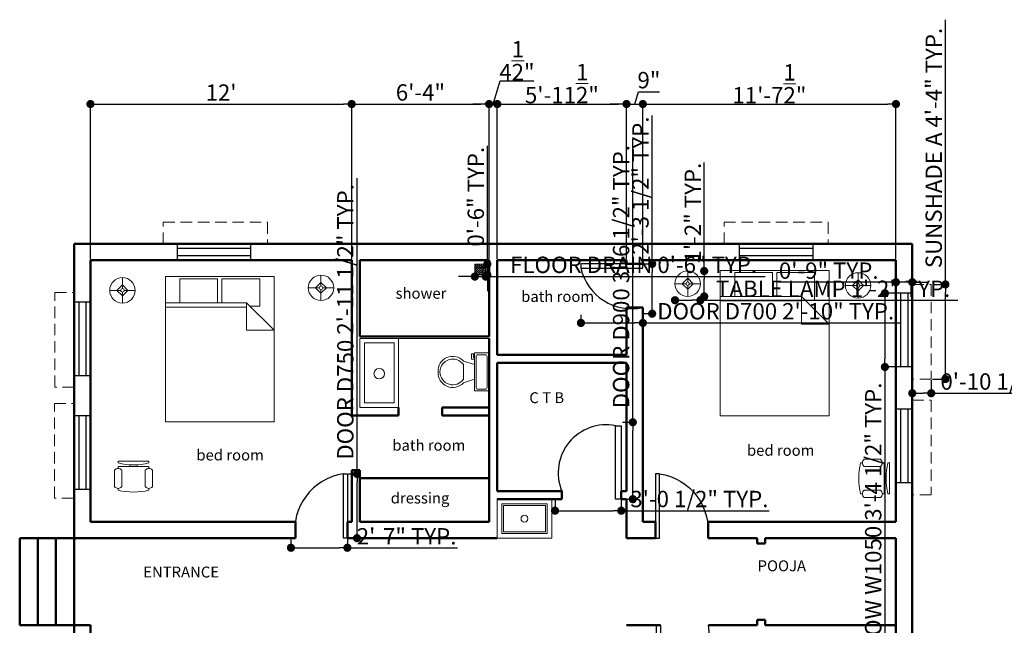
# Model space of a CAD drawing. Units: inches. Extents: x 2050 to 6806, y 2092 to 5743.
# Tile 6 of 8: x 3060 to 3602, y 2671 to 3005. Entities that reach past the tile are written whole.
import ezdxf

# ---------------------------------------------------------------- set-up
doc = ezdxf.new("R2010")
doc.units = ezdxf.units.IN
doc.linetypes.add('HIDDEN', pattern=[9.525, 6.35, -3.175])
for name, color, linetype, lineweight in [('A-ANNO-DIMS', 2, 'Continuous', 18), ('A-AREA-IDEN', 7, 'Continuous', 18), ('A-DOOR', 2, 'Continuous', 25), ('A-FLOR-FIXT', 4, 'Continuous', 18), ('A-FLOR-OVHD', 30, 'HIDDEN', 18), ('A-FURN', 5, 'Continuous', 18), ('A-GLAZ', 6, 'Continuous', 25), ('A-WALL', 7, 'Continuous', 50)]:
    doc.layers.add(name, color=color, linetype=linetype, lineweight=lineweight)
doc.styles.get("Standard").update_dxf_attribs({"font": 'arial.ttf'})
doc.dimstyles.new('ISO-25', dxfattribs={"dimtxt": 9, "dimasz": 4.5, "dimexe": 1.25, "dimexo": 0.625, "dimtad": 1, "dimdec": 1, "dimlunit": 4, "dimtxsty": 'Standard', "dimblk": 'DOT', "dimcen": 2.5, "dimadec": 0, "dimazin": 0, "dimtfac": 1, "dimtdec": 1, "dimtmove": 0, "dimatfit": 3, "dimldrblk": 'ARCHTICK', "dimfxl": 1, "dimarcsym": 0})

# ---------------------------------------------------------------- blocks, each defined once
blk = doc.blocks.new('*U4')
for p, q in [((9.5, -6), (9.5, -2)), ((-10, -8.5), (-8, -8.5)), ((-10, -9.5), (-10, -8.5)), ((-7, -9.5), (-10, -9.5)), ((-8, -8.5), (-8, -8)), ((-7, -8), (-7, -9.5)), ((-4, -8), (-6, -14)), ((4, -8), (6, -14)), ((4, -14), (-4, -14))]:
    blk.add_line(p, q)
blk.add_lwpolyline([(10.5, -8), (10.5, 0), (-10.5, 0), (-10.5, -8)], close=True)
for points in [[(-9.5, -2), (-9.5, -6)], [(8.5, -1), (-8.5, -1)], [(-8.5, -7), (8.5, -7)]]:
    blk.add_lwpolyline(points)
for centre, radius, start, end in [((-8.625, -1.875), 0.8839, 81.8699, 188.1301), ((8.625, -1.875), 0.8839, 351.8699, 98.1301), ((-8.625, -6.125), 0.8839, 171.869898, 278.1301), ((8.625, -6.125), 0.8839, 261.8699, 8.1301), ((-0.4772, -19.9188), 8.0953, 133.01722, 273.38), ((0.0374, -19.8731), 7.127, 124.50543, 269.7), ((-0.0373, -19.8731), 7.127, 270.3, 55.4946), ((0.4773, -19.9188), 8.0953, 266.62, 46.9828)]:
    blk.add_arc(centre, radius, start, end)
blk = doc.blocks.new('Bed - Queen')
for p, q in [((0, -80.00003), (0, 0)), ((0, 0), (59.99999, 0)), ((59.99999, 0), (59.99999, -80.00003)), ((7.99999, -1.2), (28.79998, -1.2)), ((7.99999, -14.4), (7.99999, -1.2)), ((28.79998, -1.2), (28.79998, -14.4)), ((31.19999, -1.2), (51.99999, -1.2)), ((31.19999, -14.4), (31.19999, -1.2)), ((51.99999, -1.2), (51.99999, -16.4)), ((0, -14.4), (44.8, -14.4)), ((59.99999, -29.6), (44.8, -14.4)), ((44.8, -14.4), (44.8, -29.6)), ((44.8, -16.8), (0, -16.8)), ((51.99999, -16.4), (46.79936, -16.4)), ((44.8, -29.6), (59.99999, -29.6)), ((59.99999, -80.00003), (0, -80.00003))]:
    blk.add_line(p, q)
blk = doc.blocks.new('Lamp - Table')
for p, q in [((0, 7), (0, 1)), ((-1, 0), (-7, 0)), ((0, 3), (-3, 0)), ((-3, 0), (0, -3)), ((3, 0), (0, 3)), ((0, -3), (3, 0)), ((1, 0), (7, 0)), ((0, -1), (0, -7))]:
    blk.add_line(p, q)
for radius in [7, 1]:
    blk.add_circle((0, 0), radius)
blk = doc.blocks.new('Chair - Desk')
for p, q in [((-8.5, 0), (-8.5, -1)), ((-8.5, 0), (8.5, 0)), ((8.5, 0), (8.5, -1)), ((-10.5, -5), (-10.5, -14)), ((-8.5, -3), (-8.5, -4)), ((-8.5, -3), (8.5, -3)), ((-6.5, -14), (-6.5, -5)), ((-2, -3), (-2, -1.9355)), ((2, -1.9576), (2, -3)), ((6.5, -5), (6.5, -14)), ((8.5, -3), (8.5, -4)), ((10.5, -14), (10.5, -5)), ((-8.5, -15), (-8.5, -16)), ((8.5, -15), (8.5, -16))]:
    blk.add_line(p, q)
for centre, radius, start, end in [((-8.5, -6.5), 2.5, 36.8699, 143.1301), ((0, 34.625), 36.625, 256.5803, 283.4197), ((8.5, -6.5), 2.5, 36.8699, 143.1301), ((-8.5, -12.5), 2.5, 216.8699, 323.1301), ((0, 19.625), 36.625, 256.5803, 283.4197), ((8.5, -12.5), 2.5, 216.8699, 323.1301)]:
    blk.add_arc(centre, radius, start, end)
blk = doc.blocks.new('_Dot')
at = {"color": 0, "linetype": 'ByBlock', "lineweight": -2}
blk.add_line((-0.5, 0), (-1, 0), dxfattribs=at)
at = {"color": 0, "linetype": 'ByBlock', "const_width": 0.5}
blk.add_lwpolyline([(-0.25, 0, 1), (0.25, 0, 1)], format="xyb", close=True, dxfattribs=at)
blk = doc.blocks.new('*D47')
at = {"layer": 'A-ANNO-DIMS', "color": 0, "lineweight": -2, "transparency": 16777216}
for p, q in [((3098.67, 2872.95), (3098.67, 2959.64)), ((3103.17, 2958.39), (3238.17, 2958.39)), ((3242.67, 2872.95), (3242.67, 2959.64))]:
    blk.add_line(p, q, dxfattribs=at)
at = {"layer": 'Defpoints', "color": 0, "transparency": 16777216}
for p in [(3242.67, 2958.39), (3098.67, 2872.33), (3242.67, 2872.33)]:
    blk.add_point(p, dxfattribs=at)
at = {"layer": 'A-ANNO-DIMS', "color": 0, "lineweight": -2, "transparency": 16777216, "xscale": 4.5, "yscale": 4.5, "zscale": 4.5, "rotation": 180}
blk.add_blockref('_Dot', (3098.67, 2958.39), dxfattribs=at)
at = {"layer": 'A-ANNO-DIMS', "color": 0, "lineweight": -2, "transparency": 16777216, "xscale": 4.5, "yscale": 4.5, "zscale": 4.5}
blk.add_blockref('_Dot', (3242.67, 2958.39), dxfattribs=at)
at = {"layer": 'A-ANNO-DIMS', "color": 0, "transparency": 16777216, "insert": (3170.67, 2963.53), "char_height": 9, "attachment_point": 5}
blk.add_mtext("12'", dxfattribs=at)
blk = doc.blocks.new('_ArchTick')
at = {"color": 0, "linetype": 'ByBlock', "const_width": 0.15}
blk.add_lwpolyline([(-0.5, -0.5), (0.5, 0.5)], dxfattribs=at)
blk = doc.blocks.new('*D48')
at = {"layer": 'A-ANNO-DIMS', "color": 0, "lineweight": -2, "transparency": 16777216}
for p, q in [((3242.67, 2872.95), (3242.67, 2959.64)), ((3247.17, 2958.39), (3313.92, 2958.39)), ((3318.42, 2872.95), (3318.42, 2959.64))]:
    blk.add_line(p, q, dxfattribs=at)
at = {"layer": 'Defpoints', "color": 0, "transparency": 16777216}
for p in [(3318.42, 2958.39), (3242.67, 2872.33), (3318.42, 2872.33)]:
    blk.add_point(p, dxfattribs=at)
at = {"layer": 'A-ANNO-DIMS', "color": 0, "lineweight": -2, "transparency": 16777216, "xscale": 4.5, "yscale": 4.5, "zscale": 4.5, "rotation": 180}
blk.add_blockref('_Dot', (3242.67, 2958.39), dxfattribs=at)
at = {"layer": 'A-ANNO-DIMS', "color": 0, "lineweight": -2, "transparency": 16777216, "xscale": 4.5, "yscale": 4.5, "zscale": 4.5}
blk.add_blockref('_Dot', (3318.42, 2958.39), dxfattribs=at)
at = {"layer": 'A-ANNO-DIMS', "color": 0, "transparency": 16777216, "insert": (3280.55, 2963.61), "char_height": 9, "attachment_point": 5}
blk.add_mtext('6\'-4"', dxfattribs=at)
blk = doc.blocks.new('*D49')
at = {"layer": 'A-ANNO-DIMS', "color": 0, "lineweight": -2, "transparency": 16777216}
for p, q in [((3320.67, 2958.39), (3324.49, 2971.11)), ((3324.49, 2971.11), (3343.01, 2971.11)), ((3313.92, 2958.39), (3309.42, 2958.39)), ((3318.42, 2872.95), (3318.42, 2959.64)), ((3318.42, 2958.39), (3322.92, 2958.39)), ((3318.42, 2958.39), (3322.92, 2958.39)), ((3322.92, 2872.95), (3322.92, 2959.64)), ((3327.42, 2958.39), (3331.92, 2958.39))]:
    blk.add_line(p, q, dxfattribs=at)
at = {"layer": 'Defpoints', "color": 0, "transparency": 16777216}
for p in [(3322.92, 2958.39), (3318.42, 2872.33), (3322.92, 2872.33)]:
    blk.add_point(p, dxfattribs=at)
at = {"layer": 'A-ANNO-DIMS', "color": 0, "lineweight": -2, "transparency": 16777216, "xscale": 4.5, "yscale": 4.5, "zscale": 4.5}
blk.add_blockref('_Dot', (3318.42, 2958.39), dxfattribs=at)
at = {"layer": 'A-ANNO-DIMS', "color": 0, "lineweight": -2, "transparency": 16777216, "xscale": 4.5, "yscale": 4.5, "zscale": 4.5, "rotation": 180}
blk.add_blockref('_Dot', (3322.92, 2958.39), dxfattribs=at)
at = {"layer": 'A-ANNO-DIMS', "color": 0, "transparency": 16777216, "insert": (3333.75, 2982.27), "char_height": 9, "attachment_point": 5}
blk.add_mtext('4{\\H1x;\\S1/2;}"', dxfattribs=at)
blk = doc.blocks.new('*D50')
at = {"layer": 'A-ANNO-DIMS', "color": 0, "lineweight": -2, "transparency": 16777216}
for p, q in [((3322.92, 2872.95), (3322.92, 2959.64)), ((3327.42, 2958.39), (3389.67, 2958.39)), ((3394.17, 2872.95), (3394.17, 2959.64))]:
    blk.add_line(p, q, dxfattribs=at)
at = {"layer": 'Defpoints', "color": 0, "transparency": 16777216}
for p in [(3394.17, 2958.39), (3322.92, 2872.33), (3394.17, 2872.33)]:
    blk.add_point(p, dxfattribs=at)
at = {"layer": 'A-ANNO-DIMS', "color": 0, "lineweight": -2, "transparency": 16777216, "xscale": 4.5, "yscale": 4.5, "zscale": 4.5, "rotation": 180}
blk.add_blockref('_Dot', (3322.92, 2958.39), dxfattribs=at)
at = {"layer": 'A-ANNO-DIMS', "color": 0, "lineweight": -2, "transparency": 16777216, "xscale": 4.5, "yscale": 4.5, "zscale": 4.5}
blk.add_blockref('_Dot', (3394.17, 2958.39), dxfattribs=at)
at = {"layer": 'A-ANNO-DIMS', "color": 0, "transparency": 16777216, "insert": (3358.55, 2969.62), "char_height": 9, "attachment_point": 5}
blk.add_mtext('5\'-11{\\H1x;\\S1/2;}"', dxfattribs=at)
blk = doc.blocks.new('*D51')
at = {"layer": 'A-ANNO-DIMS', "color": 0, "lineweight": -2, "transparency": 16777216}
for p, q in [((3398.67, 2958.39), (3400.71, 2965.17)), ((3400.71, 2965.17), (3412.3, 2965.17)), ((3389.67, 2958.39), (3385.17, 2958.39)), ((3394.17, 2872.95), (3394.17, 2959.64)), ((3394.17, 2958.39), (3403.17, 2958.39)), ((3394.17, 2958.39), (3403.17, 2958.39)), ((3403.17, 2872.95), (3403.17, 2959.64)), ((3407.67, 2958.39), (3412.17, 2958.39))]:
    blk.add_line(p, q, dxfattribs=at)
at = {"layer": 'Defpoints', "color": 0, "transparency": 16777216}
for p in [(3403.17, 2958.39), (3394.17, 2872.33), (3403.17, 2872.33)]:
    blk.add_point(p, dxfattribs=at)
at = {"layer": 'A-ANNO-DIMS', "color": 0, "lineweight": -2, "transparency": 16777216, "xscale": 4.5, "yscale": 4.5, "zscale": 4.5}
blk.add_blockref('_Dot', (3394.17, 2958.39), dxfattribs=at)
at = {"layer": 'A-ANNO-DIMS', "color": 0, "lineweight": -2, "transparency": 16777216, "xscale": 4.5, "yscale": 4.5, "zscale": 4.5, "rotation": 180}
blk.add_blockref('_Dot', (3403.17, 2958.39), dxfattribs=at)
at = {"layer": 'A-ANNO-DIMS', "color": 0, "transparency": 16777216, "insert": (3406.5, 2970.39), "char_height": 9, "attachment_point": 5}
blk.add_mtext('9"', dxfattribs=at)
blk = doc.blocks.new('*D52')
at = {"layer": 'A-ANNO-DIMS', "color": 0, "lineweight": -2, "transparency": 16777216}
for p, q in [((3403.17, 2872.95), (3403.17, 2959.64)), ((3407.67, 2958.39), (3538.17, 2958.39)), ((3542.67, 2872.95), (3542.67, 2959.64))]:
    blk.add_line(p, q, dxfattribs=at)
at = {"layer": 'Defpoints', "color": 0, "transparency": 16777216}
for p in [(3542.67, 2958.39), (3403.17, 2872.33), (3542.67, 2872.33)]:
    blk.add_point(p, dxfattribs=at)
at = {"layer": 'A-ANNO-DIMS', "color": 0, "lineweight": -2, "transparency": 16777216, "xscale": 4.5, "yscale": 4.5, "zscale": 4.5, "rotation": 180}
blk.add_blockref('_Dot', (3403.17, 2958.39), dxfattribs=at)
at = {"layer": 'A-ANNO-DIMS', "color": 0, "lineweight": -2, "transparency": 16777216, "xscale": 4.5, "yscale": 4.5, "zscale": 4.5}
blk.add_blockref('_Dot', (3542.67, 2958.39), dxfattribs=at)
at = {"layer": 'A-ANNO-DIMS', "color": 0, "transparency": 16777216, "insert": (3472.92, 2969.55), "char_height": 9, "attachment_point": 5}
blk.add_mtext('11\'-7{\\H1x;\\S1/2;}"', dxfattribs=at)
blk = doc.blocks.new('DOOR-750')
blk.add_lwpolyline([(28.97, 0), (26.83, 0), (26.83, 35.38), (28.97, 35.38)], close=True)
blk.add_arc((31.25, 4.42), 31.27, 98.1233, 188.1233)
blk = doc.blocks.new('DOOR-700')
blk.add_lwpolyline([(34.15, 24.67), (0, 24.67), (0, 22.42), (34.15, 22.42)], close=True)
blk.add_arc((27.99, 28.69), 28.69, 192.6316, 282.383)
blk = doc.blocks.new('DOOR-900')
blk.add_lwpolyline([(34.8, 0), (31.58, 0), (31.58, 40.43), (34.8, 40.43)], close=True)
blk.add_arc((26.4, 14.55), 26.4, 78.6709, 202.3636)
blk = doc.blocks.new('WIN-1050')
for p, q in [((0, 40.58), (9, 40.58)), ((2.5, 0), (2.5, 40.58)), ((6.5, 0), (6.5, 40.58)), ((0, 0), (9, 0))]:
    blk.add_line(p, q)
blk = doc.blocks.new('SUNSHADE-A')
for p, q in [((0, 52.08), (10.45, 52.08)), ((10.45, 52.08), (10.45, 0)), ((10.45, 0), (0, 0))]:
    blk.add_line(p, q)
blk = doc.blocks.new('SUNSHADE-B')
for p, q in [((0, 0), (0, 11.94)), ((0, 11.94), (57.41, 11.94)), ((57.41, 11.94), (57.41, 0.04))]:
    blk.add_line(p, q)
blk = doc.blocks.new('FLOOR-DRAIN')
blk.add_lwpolyline([(0, 0), (6, 0), (6, 6), (0, 6)], close=True)
for centre in [(0.84, 5.43), (1.9, 5.43), (3.09, 5.43), (4.24, 5.43), (5.33, 5.43), (0.84, 4.34), (0.84, 3.14), (0.84, 1.97), (0.84, 0.74), (2.07, 4.34), (2.07, 3.14), (2.07, 1.97), (2.07, 0.74), (3.3, 4.34), (3.3, 3.14), (3.3, 1.97), (3.3, 0.74), (4.49, 4.34), (4.49, 3.14), (4.49, 1.97), (4.49, 0.74), (5.5, 4.34), (5.5, 3.14), (5.5, 1.97), (5.5, 0.74)]:
    blk.add_circle(centre, 0.471)
blk = doc.blocks.new('WASHBASIN')
blk.add_lwpolyline([(16.37, 33), (16.37, 0), (0, 0), (0, 33)], close=True)
blk.add_circle((8.19, 16.05), 2.91)
blk = doc.blocks.new('*D67')
at = {"layer": 'A-ANNO-DIMS', "color": 0, "lineweight": -2, "transparency": 16777216}
for p, q in [((3542.05, 2854.17), (3535.33, 2854.17)), ((3536.58, 2849.67), (3536.58, 2818.09)), ((3542.05, 2813.59), (3535.33, 2813.59)), ((3536.58, 2813.59), (3536.58, 2629.65))]:
    blk.add_line(p, q, dxfattribs=at)
at = {"layer": 'Defpoints', "color": 0, "transparency": 16777216}
for p in [(3542.67, 2854.17), (3536.58, 2813.59), (3542.67, 2813.59)]:
    blk.add_point(p, dxfattribs=at)
at = {"layer": 'A-ANNO-DIMS', "color": 0, "lineweight": -2, "transparency": 16777216, "xscale": 4.5, "yscale": 4.5, "zscale": 4.5}
for p, rotation in [((3536.58, 2854.17), 90), ((3536.58, 2813.59), 270)]:
    blk.add_blockref('_Dot', p, dxfattribs=dict(at, rotation=rotation))
at = {"layer": 'A-ANNO-DIMS', "color": 0, "transparency": 16777216, "insert": (3531.3, 2719.37), "char_height": 9, "attachment_point": 5, "rotation": 90}
blk.add_mtext('WINDOW W1050 3\'-4 1/2" TYP.', dxfattribs=at)
blk = doc.blocks.new('*D68')
at = {"layer": 'A-ANNO-DIMS', "color": 0, "lineweight": -2, "transparency": 16777216}
for p, q in [((3538.17, 2860.26), (3477.56, 2860.26)), ((3542.67, 2854.8), (3542.67, 2861.51)), ((3551.67, 2860.26), (3542.67, 2860.26)), ((3551.67, 2854.8), (3551.67, 2861.51)), ((3556.17, 2860.26), (3560.67, 2860.26))]:
    blk.add_line(p, q, dxfattribs=at)
at = {"layer": 'Defpoints', "color": 0, "transparency": 16777216}
for p in [(3542.67, 2860.26), (3542.67, 2854.17), (3551.67, 2854.17)]:
    blk.add_point(p, dxfattribs=at)
at = {"layer": 'A-ANNO-DIMS', "color": 0, "lineweight": -2, "transparency": 16777216, "xscale": 4.5, "yscale": 4.5, "zscale": 4.5}
blk.add_blockref('_Dot', (3542.67, 2860.26), dxfattribs=at)
at = {"layer": 'A-ANNO-DIMS', "color": 0, "lineweight": -2, "transparency": 16777216, "xscale": 4.5, "yscale": 4.5, "zscale": 4.5, "rotation": 180}
blk.add_blockref('_Dot', (3551.67, 2860.26), dxfattribs=at)
at = {"layer": 'A-ANNO-DIMS', "color": 0, "transparency": 16777216, "insert": (3505.62, 2865.48), "char_height": 9, "attachment_point": 5}
blk.add_mtext('0\'-9" TYP.', dxfattribs=at)
blk = doc.blocks.new('*D71')
at = {"layer": 'A-ANNO-DIMS', "color": 0, "lineweight": -2, "transparency": 16777216}
for p, q in [((3245.61, 2754.7), (3245.61, 2917.59)), ((3240.92, 2754.7), (3246.86, 2754.7)), ((3245.61, 2723.83), (3245.61, 2750.2)), ((3240.92, 2719.33), (3246.86, 2719.33))]:
    blk.add_line(p, q, dxfattribs=at)
at = {"layer": 'Defpoints', "color": 0, "transparency": 16777216}
for p in [(3240.3, 2754.7), (3245.61, 2754.7), (3240.3, 2719.33)]:
    blk.add_point(p, dxfattribs=at)
at = {"layer": 'A-ANNO-DIMS', "color": 0, "lineweight": -2, "transparency": 16777216, "xscale": 4.5, "yscale": 4.5, "zscale": 4.5}
for p, rotation in [((3245.61, 2754.7), 90), ((3245.61, 2719.33), 270)]:
    blk.add_blockref('_Dot', p, dxfattribs=dict(at, rotation=rotation))
at = {"layer": 'A-ANNO-DIMS', "color": 0, "transparency": 16777216, "insert": (3240.32, 2838.4), "char_height": 9, "attachment_point": 5, "rotation": 90}
blk.add_mtext('DOOR D750 2\'-11 1/2" TYP.', dxfattribs=at)
blk = doc.blocks.new('*D72')
at = {"layer": 'A-ANNO-DIMS', "color": 0, "lineweight": -2, "transparency": 16777216}
for p, q in [((3209.18, 2718.7), (3209.18, 2712.77)), ((3213.68, 2714.02), (3235.8, 2714.02)), ((3240.3, 2718.7), (3240.3, 2712.77)), ((3240.3, 2714.02), (3301.06, 2714.02))]:
    blk.add_line(p, q, dxfattribs=at)
at = {"layer": 'Defpoints', "color": 0, "transparency": 16777216}
for p in [(3209.18, 2719.33), (3240.3, 2719.33), (3240.3, 2714.02)]:
    blk.add_point(p, dxfattribs=at)
at = {"layer": 'A-ANNO-DIMS', "color": 0, "lineweight": -2, "transparency": 16777216, "xscale": 4.5, "yscale": 4.5, "zscale": 4.5, "rotation": 180}
blk.add_blockref('_Dot', (3209.18, 2714.02), dxfattribs=at)
at = {"layer": 'A-ANNO-DIMS', "color": 0, "lineweight": -2, "transparency": 16777216, "xscale": 4.5, "yscale": 4.5, "zscale": 4.5}
blk.add_blockref('_Dot', (3240.3, 2714.02), dxfattribs=at)
at = {"layer": 'A-ANNO-DIMS', "color": 0, "transparency": 16777216, "insert": (3272.93, 2719.17), "char_height": 9, "attachment_point": 5}
blk.add_mtext('2\'-7" TYP.', dxfattribs=at)
blk = doc.blocks.new('*D73')
at = {"layer": 'A-ANNO-DIMS', "color": 0, "lineweight": -2, "transparency": 16777216}
for p, q in [((3369.03, 2842.32), (3369.03, 2836.58)), ((3403.17, 2842.32), (3403.17, 2836.58)), ((3373.53, 2837.83), (3398.67, 2837.83)), ((3403.17, 2837.83), (3545.09, 2837.83))]:
    blk.add_line(p, q, dxfattribs=at)
at = {"layer": 'Defpoints', "color": 0, "transparency": 16777216}
for p in [(3369.03, 2842.95), (3403.17, 2842.95), (3403.17, 2837.83)]:
    blk.add_point(p, dxfattribs=at)
at = {"layer": 'A-ANNO-DIMS', "color": 0, "lineweight": -2, "transparency": 16777216, "xscale": 4.5, "yscale": 4.5, "zscale": 4.5, "rotation": 180}
blk.add_blockref('_Dot', (3369.03, 2837.83), dxfattribs=at)
at = {"layer": 'A-ANNO-DIMS', "color": 0, "lineweight": -2, "transparency": 16777216, "xscale": 4.5, "yscale": 4.5, "zscale": 4.5}
blk.add_blockref('_Dot', (3403.17, 2837.83), dxfattribs=at)
at = {"layer": 'A-ANNO-DIMS', "color": 0, "transparency": 16777216, "insert": (3476.38, 2843.11), "char_height": 9, "attachment_point": 5}
blk.add_mtext('DOOR D700 2\'-10" TYP.', dxfattribs=at)
blk = doc.blocks.new('*D74')
at = {"layer": 'A-ANNO-DIMS', "color": 0, "lineweight": -2, "transparency": 16777216}
for p, q in [((3408.29, 2870.34), (3408.29, 2952.07)), ((3403.8, 2870.34), (3409.54, 2870.34)), ((3408.29, 2847.45), (3408.29, 2865.84)), ((3403.8, 2842.95), (3409.54, 2842.95))]:
    blk.add_line(p, q, dxfattribs=at)
at = {"layer": 'Defpoints', "color": 0, "transparency": 16777216}
for p in [(3403.17, 2870.34), (3408.29, 2870.34), (3403.17, 2842.95)]:
    blk.add_point(p, dxfattribs=at)
at = {"layer": 'A-ANNO-DIMS', "color": 0, "lineweight": -2, "transparency": 16777216, "xscale": 4.5, "yscale": 4.5, "zscale": 4.5}
for p, rotation in [((3408.29, 2870.34), 90), ((3408.29, 2842.95), 270)]:
    blk.add_blockref('_Dot', p, dxfattribs=dict(at, rotation=rotation))
at = {"layer": 'A-ANNO-DIMS', "color": 0, "transparency": 16777216, "insert": (3403.01, 2913.45), "char_height": 9, "attachment_point": 5, "rotation": 90}
blk.add_mtext('2\'-3 1/2" TYP.', dxfattribs=at)
blk = doc.blocks.new('*D75')
at = {"layer": 'A-ANNO-DIMS', "color": 0, "lineweight": -2, "transparency": 16777216}
for p, q in [((3397.63, 2783.13), (3397.63, 2939.02)), ((3391.91, 2783.13), (3398.88, 2783.13)), ((3397.63, 2745.28), (3397.63, 2778.63)), ((3391.91, 2740.78), (3398.88, 2740.78))]:
    blk.add_line(p, q, dxfattribs=at)
at = {"layer": 'Defpoints', "color": 0, "transparency": 16777216}
for p in [(3391.28, 2783.13), (3397.63, 2783.13), (3391.28, 2740.78)]:
    blk.add_point(p, dxfattribs=at)
at = {"layer": 'A-ANNO-DIMS', "color": 0, "lineweight": -2, "transparency": 16777216, "xscale": 4.5, "yscale": 4.5, "zscale": 4.5}
for p, rotation in [((3397.63, 2783.13), 90), ((3397.63, 2740.78), 270)]:
    blk.add_blockref('_Dot', p, dxfattribs=dict(at, rotation=rotation))
at = {"layer": 'A-ANNO-DIMS', "color": 0, "transparency": 16777216, "insert": (3392.35, 2863.32), "char_height": 9, "attachment_point": 5, "rotation": 90}
blk.add_mtext('DOOR D900 3\'-6 1/2" TYP.', dxfattribs=at)
blk = doc.blocks.new('*D76')
at = {"layer": 'A-ANNO-DIMS', "color": 0, "lineweight": -2, "transparency": 16777216}
for p, q in [((3354.76, 2740.16), (3354.76, 2733.18)), ((3391.28, 2740.16), (3391.28, 2733.18)), ((3359.26, 2734.43), (3386.78, 2734.43)), ((3391.28, 2734.43), (3472.86, 2734.43))]:
    blk.add_line(p, q, dxfattribs=at)
at = {"layer": 'Defpoints', "color": 0, "transparency": 16777216}
for p in [(3354.76, 2740.78), (3391.28, 2740.78), (3391.28, 2734.43)]:
    blk.add_point(p, dxfattribs=at)
at = {"layer": 'A-ANNO-DIMS', "color": 0, "lineweight": -2, "transparency": 16777216, "xscale": 4.5, "yscale": 4.5, "zscale": 4.5, "rotation": 180}
blk.add_blockref('_Dot', (3354.76, 2734.43), dxfattribs=at)
at = {"layer": 'A-ANNO-DIMS', "color": 0, "lineweight": -2, "transparency": 16777216, "xscale": 4.5, "yscale": 4.5, "zscale": 4.5}
blk.add_blockref('_Dot', (3391.28, 2734.43), dxfattribs=at)
at = {"layer": 'A-ANNO-DIMS', "color": 0, "transparency": 16777216, "insert": (3434.32, 2739.71), "char_height": 9, "attachment_point": 5}
blk.add_mtext('3\'-0 1/2" TYP.', dxfattribs=at)
blk = doc.blocks.new('*D79')
at = {"layer": 'A-ANNO-DIMS', "color": 0, "lineweight": -2, "transparency": 16777216}
for p, q in [((3569.93, 2859.03), (3569.93, 3004.83)), ((3562.74, 2859.03), (3571.18, 2859.03)), ((3569.93, 2811.45), (3569.93, 2854.53)), ((3562.74, 2806.95), (3571.18, 2806.95))]:
    blk.add_line(p, q, dxfattribs=at)
at = {"layer": 'Defpoints', "color": 0, "transparency": 16777216}
for p in [(3562.12, 2859.03), (3569.93, 2859.03), (3562.12, 2806.95)]:
    blk.add_point(p, dxfattribs=at)
at = {"layer": 'A-ANNO-DIMS', "color": 0, "lineweight": -2, "transparency": 16777216, "xscale": 4.5, "yscale": 4.5, "zscale": 4.5}
for p, rotation in [((3569.93, 2859.03), 90), ((3569.93, 2806.95), 270)]:
    blk.add_blockref('_Dot', p, dxfattribs=dict(at, rotation=rotation))
at = {"layer": 'A-ANNO-DIMS', "color": 0, "transparency": 16777216, "insert": (3564.65, 2934.18), "char_height": 9, "attachment_point": 5, "rotation": 90}
blk.add_mtext('SUNSHADE A 4\'-4" TYP.', dxfattribs=at)
blk = doc.blocks.new('*D80')
at = {"layer": 'A-ANNO-DIMS', "color": 0, "lineweight": -2, "transparency": 16777216}
for p, q in [((3551.67, 2806.32), (3551.67, 2797.88)), ((3562.12, 2806.32), (3562.12, 2797.88)), ((3556.17, 2799.13), (3557.62, 2799.13)), ((3562.12, 2799.13), (3650.69, 2799.13))]:
    blk.add_line(p, q, dxfattribs=at)
at = {"layer": 'Defpoints', "color": 0, "transparency": 16777216}
for p in [(3551.67, 2806.95), (3562.12, 2806.95), (3562.12, 2799.13)]:
    blk.add_point(p, dxfattribs=at)
at = {"layer": 'A-ANNO-DIMS', "color": 0, "lineweight": -2, "transparency": 16777216, "xscale": 4.5, "yscale": 4.5, "zscale": 4.5, "rotation": 180}
blk.add_blockref('_Dot', (3551.67, 2799.13), dxfattribs=at)
at = {"layer": 'A-ANNO-DIMS', "color": 0, "lineweight": -2, "transparency": 16777216, "xscale": 4.5, "yscale": 4.5, "zscale": 4.5}
blk.add_blockref('_Dot', (3562.12, 2799.13), dxfattribs=at)
at = {"layer": 'A-ANNO-DIMS', "color": 0, "transparency": 16777216, "insert": (3608.66, 2804.41), "char_height": 9, "attachment_point": 5}
blk.add_mtext('0\'-10 1/2" TYP.', dxfattribs=at)
blk = doc.blocks.new('*D87')
at = {"layer": 'A-ANNO-DIMS', "color": 0, "lineweight": -2, "transparency": 16777216}
for p, q in [((3420.88, 2851.82), (3420.88, 2849.09)), ((3425.38, 2850.34), (3430.38, 2850.34)), ((3434.88, 2851.82), (3434.88, 2849.09)), ((3434.88, 2850.34), (3576.77, 2850.34))]:
    blk.add_line(p, q, dxfattribs=at)
at = {"layer": 'Defpoints', "color": 0, "transparency": 16777216}
for p in [(3420.88, 2852.44), (3434.88, 2852.44), (3434.88, 2850.34)]:
    blk.add_point(p, dxfattribs=at)
at = {"layer": 'A-ANNO-DIMS', "color": 0, "lineweight": -2, "transparency": 16777216, "xscale": 4.5, "yscale": 4.5, "zscale": 4.5, "rotation": 180}
blk.add_blockref('_Dot', (3420.88, 2850.34), dxfattribs=at)
at = {"layer": 'A-ANNO-DIMS', "color": 0, "lineweight": -2, "transparency": 16777216, "xscale": 4.5, "yscale": 4.5, "zscale": 4.5}
blk.add_blockref('_Dot', (3434.88, 2850.34), dxfattribs=at)
at = {"layer": 'A-ANNO-DIMS', "color": 0, "transparency": 16777216, "insert": (3508.08, 2855.49), "char_height": 9, "attachment_point": 5}
blk.add_mtext('TABLE LAMP 1\'-2" TYP.', dxfattribs=at)
blk = doc.blocks.new('*D88')
at = {"layer": 'A-ANNO-DIMS', "color": 0, "lineweight": -2, "transparency": 16777216}
for p, q in [((3436.98, 2866.44), (3436.98, 2926.21)), ((3435.51, 2866.44), (3438.23, 2866.44)), ((3436.98, 2856.94), (3436.98, 2861.94)), ((3435.51, 2852.44), (3438.23, 2852.44))]:
    blk.add_line(p, q, dxfattribs=at)
at = {"layer": 'Defpoints', "color": 0, "transparency": 16777216}
for p in [(3434.88, 2866.44), (3436.98, 2866.44), (3434.88, 2852.44)]:
    blk.add_point(p, dxfattribs=at)
at = {"layer": 'A-ANNO-DIMS', "color": 0, "lineweight": -2, "transparency": 16777216, "xscale": 4.5, "yscale": 4.5, "zscale": 4.5}
for p, rotation in [((3436.98, 2866.44), 90), ((3436.98, 2852.44), 270)]:
    blk.add_blockref('_Dot', p, dxfattribs=dict(at, rotation=rotation))
at = {"layer": 'A-ANNO-DIMS', "color": 0, "transparency": 16777216, "insert": (3431.84, 2898.58), "char_height": 9, "attachment_point": 5, "rotation": 90}
blk.add_mtext('1\'-2" TYP.', dxfattribs=at)
blk = doc.blocks.new('*D101')
at = {"layer": 'A-ANNO-DIMS', "color": 0, "lineweight": -2, "transparency": 16777216}
for p, q in [((3306.05, 2863.37), (3301.55, 2863.37)), ((3310.55, 2863.65), (3310.55, 2862.12)), ((3310.55, 2863.37), (3316.55, 2863.37)), ((3316.55, 2863.65), (3316.55, 2862.12)), ((3321.05, 2863.37), (3470.57, 2863.37))]:
    blk.add_line(p, q, dxfattribs=at)
at = {"layer": 'Defpoints', "color": 0, "transparency": 16777216}
for p in [(3310.55, 2864.27), (3316.55, 2864.27), (3316.55, 2863.37)]:
    blk.add_point(p, dxfattribs=at)
at = {"layer": 'A-ANNO-DIMS', "color": 0, "lineweight": -2, "transparency": 16777216, "xscale": 4.5, "yscale": 4.5, "zscale": 4.5}
blk.add_blockref('_Dot', (3310.55, 2863.37), dxfattribs=at)
at = {"layer": 'A-ANNO-DIMS', "color": 0, "lineweight": -2, "transparency": 16777216, "xscale": 4.5, "yscale": 4.5, "zscale": 4.5, "rotation": 180}
blk.add_blockref('_Dot', (3316.55, 2863.37), dxfattribs=at)
at = {"layer": 'A-ANNO-DIMS', "color": 0, "transparency": 16777216, "insert": (3398.06, 2868.66), "char_height": 9, "attachment_point": 5}
blk.add_mtext('FLOOR DRAIN 0\'-6" TYP.', dxfattribs=at)
blk = doc.blocks.new('*D102')
at = {"layer": 'A-ANNO-DIMS', "color": 0, "lineweight": -2, "transparency": 16777216}
for p, q in [((3317.45, 2874.77), (3317.45, 2935.38)), ((3317.18, 2870.27), (3318.7, 2870.27)), ((3317.45, 2864.27), (3317.45, 2870.27)), ((3317.18, 2864.27), (3318.7, 2864.27)), ((3317.45, 2859.77), (3317.45, 2855.27))]:
    blk.add_line(p, q, dxfattribs=at)
at = {"layer": 'Defpoints', "color": 0, "transparency": 16777216}
for p in [(3316.55, 2870.27), (3317.45, 2870.27), (3316.55, 2864.27)]:
    blk.add_point(p, dxfattribs=at)
at = {"layer": 'A-ANNO-DIMS', "color": 0, "lineweight": -2, "transparency": 16777216, "xscale": 4.5, "yscale": 4.5, "zscale": 4.5}
for p, rotation in [((3317.45, 2870.27), 270), ((3317.45, 2864.27), 90)]:
    blk.add_blockref('_Dot', p, dxfattribs=dict(at, rotation=rotation))
at = {"layer": 'A-ANNO-DIMS', "color": 0, "transparency": 16777216, "insert": (3312.23, 2907.33), "char_height": 9, "attachment_point": 5, "rotation": 90}
blk.add_mtext('0\'-6" TYP.', dxfattribs=at)

msp = doc.modelspace()

# ---------------------------------------------------------------- linework, layer by layer
at = {"layer": 'A-FLOR-FIXT'}
for p, q in [((3322.92, 2740.78), (3322.92, 2719.33)), ((3350.42, 2738.28), (3325.42, 2738.28)), ((3325.42, 2738.28), (3325.42, 2721.83)), ((3349.42, 2737.28), (3326.42, 2737.28)), ((3326.42, 2737.28), (3326.42, 2722.83)), ((3349.42, 2737.28), (3349.42, 2722.83)), ((3350.42, 2738.28), (3350.42, 2721.83)), ((3352.92, 2740.78), (3352.92, 2719.33)), ((3322.92, 2719.33), (3352.92, 2719.33)), ((3325.42, 2721.83), (3350.42, 2721.83)), ((3326.42, 2722.83), (3349.42, 2722.83))]:
    msp.add_line(p, q, dxfattribs=at)
msp.add_lwpolyline([(3268.55, 2829.33), (3268.55, 2791.33), (3247.17, 2791.33), (3247.17, 2829.33), (3318.42, 2829.33)], dxfattribs=at)
msp.add_circle((3337.92, 2730.05), 1.9, dxfattribs=at)
at = {"layer": 'A-WALL'}
for p, q in [((3551.67, 2881.33), (3089.67, 2881.33)), ((3089.67, 2881.33), (3089.67, 2719.33)), ((3551.67, 2416.33), (3551.67, 2881.33)), ((3242.67, 2872.33), (3098.67, 2872.33)), ((3098.67, 2872.33), (3098.67, 2728.33)), ((3242.67, 2872.33), (3242.67, 2786.83)), ((3318.42, 2872.33), (3247.17, 2872.33)), ((3247.17, 2872.33), (3247.17, 2830.33)), ((3318.42, 2872.33), (3318.42, 2830.33)), ((3394.17, 2872.33), (3322.92, 2872.33)), ((3322.92, 2872.33), (3322.92, 2820.35)), ((3394.17, 2870.34), (3394.17, 2872.33)), ((3403.17, 2870.34), (3403.17, 2872.33)), ((3542.67, 2872.33), (3403.17, 2872.33)), ((3542.67, 2728.33), (3542.67, 2872.33)), ((3394.17, 2870.34), (3403.17, 2870.34)), ((3394.17, 2820.35), (3394.17, 2846.34)), ((3394.17, 2846.34), (3403.17, 2846.34)), ((3403.17, 2728.33), (3403.17, 2846.34)), ((3318.42, 2830.33), (3247.17, 2830.33)), ((3318.42, 2829.33), (3318.42, 2728.33)), ((3394.17, 2820.35), (3322.92, 2820.35)), ((3394.17, 2815.85), (3322.92, 2815.85)), ((3322.92, 2815.85), (3322.92, 2805.65)), ((3322.92, 2815.85), (3322.92, 2745.28)), ((3394.17, 2805.65), (3394.17, 2815.85)), ((3394.17, 2795.48), (3394.17, 2815.85)), ((3394.17, 2805.65), (3394.17, 2815.85)), ((3394.17, 2745.28), (3394.17, 2801.15)), ((3403.17, 2728.33), (3403.17, 2801.15)), ((3268.55, 2791.33), (3268.55, 2786.83)), ((3318.42, 2791.33), (3292.55, 2791.33)), ((3292.55, 2791.33), (3292.55, 2786.83)), ((3268.55, 2786.83), (3242.67, 2786.83)), ((3318.42, 2786.83), (3292.55, 2786.83)), ((3247.17, 2756.83), (3242.67, 2756.83)), ((3242.67, 2756.83), (3242.67, 2728.33)), ((3247.17, 2756.83), (3247.17, 2728.33)), ((3318.42, 2752.33), (3247.17, 2752.33)), ((3358.47, 2745.28), (3322.92, 2745.28)), ((3358.47, 2745.28), (3358.47, 2740.78)), ((3394.17, 2745.28), (3391.28, 2745.28)), ((3391.28, 2745.28), (3391.28, 2740.78)), ((3358.47, 2740.78), (3322.92, 2740.78)), ((3394.17, 2740.78), (3391.28, 2740.78)), ((3394.17, 2719.33), (3394.17, 2740.78)), ((3211.62, 2728.33), (3098.67, 2728.33)), ((3211.62, 2728.33), (3211.62, 2719.33)), ((3211.62, 2728.33), (3211.62, 2719.33)), ((3211.62, 2728.33), (3211.62, 2719.33)), ((3242.67, 2728.33), (3240.3, 2728.33)), ((3240.3, 2728.33), (3240.3, 2719.33)), ((3240.3, 2728.33), (3240.3, 2719.33)), ((3318.42, 2728.33), (3247.17, 2728.33)), ((3410.18, 2728.33), (3403.17, 2728.33)), ((3410.18, 2728.33), (3410.18, 2719.33)), ((3542.67, 2728.33), (3439.17, 2728.33)), ((3439.17, 2728.33), (3439.17, 2719.33)), ((3059.67, 2671.33), (3059.67, 2719.33)), ((3059.67, 2719.33), (3089.67, 2719.33)), ((3069.67, 2671.33), (3069.67, 2719.33)), ((3079.67, 2671.33), (3079.67, 2719.33)), ((3211.62, 2719.33), (3089.67, 2719.33)), ((3089.67, 2671.33), (3089.67, 2719.33)), ((3322.92, 2719.33), (3240.3, 2719.33)), ((3410.18, 2719.33), (3394.17, 2719.33)), ((3466.17, 2719.33), (3439.17, 2719.33)), ((3466.17, 2716.33), (3466.17, 2719.33)), ((3470.67, 2716.33), (3470.67, 2719.33)), ((3542.67, 2719.33), (3470.67, 2719.33)), ((3542.67, 2546.83), (3542.67, 2719.33)), ((3470.67, 2716.33), (3466.17, 2716.33)), ((3059.67, 2671.33), (3089.67, 2671.33)), ((3089.67, 2671.33), (3089.67, 2347.33)), ((3098.67, 2671.33), (3089.67, 2671.33)), ((3098.67, 2671.33), (3098.67, 2356.33)), ((3412.81, 2671.33), (3394.17, 2671.33)), ((3466.17, 2671.33), (3439.35, 2671.33)), ((3466.17, 2671.33), (3451.17, 2671.33)), ((3466.17, 2671.33), (3466.17, 2674.33)), ((3466.17, 2674.33), (3470.67, 2674.33)), ((3470.67, 2671.33), (3470.67, 2674.33)), ((3542.67, 2671.33), (3470.67, 2671.33))]:
    msp.add_line(p, q, dxfattribs=at)

# ---------------------------------------------------------------- block references
at = {"layer": 'A-DOOR'}
for name, p in [('DOOR-700', (3369.02, 2845.67)), ('DOOR-900', (3356.49, 2740.78)), ('DOOR-750', (3211.33, 2719.33))]:
    msp.add_blockref(name, p, dxfattribs=at)
at = {"layer": 'A-DOOR', "extrusion": (0, 0, -1), "zscale": -1}
msp.add_blockref('DOOR-750', (-3439.14, 2719.33), dxfattribs=at)
at = {"layer": 'A-DOOR', "rotation": 180}
msp.add_blockref('DOOR-750', (3439.64, 2671.33), dxfattribs=at)
at = {"layer": 'A-FLOR-FIXT'}
for name, p in [('FLOOR-DRAIN', (3310.55, 2864.27)), ('WASHBASIN', (3249.67, 2793.83))]:
    msp.add_blockref(name, p, dxfattribs=at)
at = {"layer": 'A-FLOR-FIXT', "rotation": 270}
msp.add_blockref('*U4', (3318.28, 2810.86), dxfattribs=at)
at = {"layer": 'A-FLOR-OVHD'}
for name, p in [('SUNSHADE-B', (3138.84, 2881.33)), ('SUNSHADE-B', (3447.94, 2881.33)), ('SUNSHADE-A', (3551.67, 2806.95)), ('SUNSHADE-A', (3551.67, 2743.21))]:
    msp.add_blockref(name, p, dxfattribs=at)
at = {"layer": 'A-FLOR-OVHD', "rotation": 180}
for p in [(3089.58, 2854.53), (3089.23, 2793.48)]:
    msp.add_blockref('SUNSHADE-A', p, dxfattribs=at)
at = {"layer": 'A-FURN'}
for name, p in [('Lamp - Table', (3427.88, 2859.44)), ('Bed - Queen', (3445.82, 2866.75)), ('Lamp - Table', (3116.29, 2855.77)), ('Bed - Queen', (3139.97, 2863.39)), ('Lamp - Table', (3225.75, 2857.18)), ('Lamp - Table', (3521.8, 2858.51)), ('Chair - Desk', (3122.4, 2761.71))]:
    msp.add_blockref(name, p, dxfattribs=at)
at = {"layer": 'A-FURN', "rotation": 270}
msp.add_blockref('Chair - Desk', (3539.19, 2752.23), dxfattribs=at)
at = {"layer": 'A-GLAZ'}
for p, rotation in [((3187.17, 2872.37), 90.00000000000246), ((3496.97, 2872.25), 90.00000000000273), ((3551.67, 2854.17), 180), ((3098.69, 2849.21), 180), ((3551.67, 2790.33), 180), ((3098.69, 2786.66), 180)]:
    msp.add_blockref('WIN-1050', p, dxfattribs=dict(at, rotation=rotation))

# ---------------------------------------------------------------- texts
at = {"layer": 'A-AREA-IDEN'}
for s, p in [('shower', (3266.84, 2851.17)), ('bath room', (3336.09, 2849.41)), ('C T B ', (3340.58, 2793.66)), ('bath room', (3265.08, 2767.48)), ('bed room', (3157.07, 2762.11)), ('bed room', (3460.56, 2764.68)), ('dressing ', (3264.2, 2738.41)), ('ENTRANCE', (3127.78, 2697.66)), ('POOJA', (3466.43, 2701.08))]:
    msp.add_text(s, height=6, dxfattribs=at).set_placement(p)

# ---------------------------------------------------------------- dimensions: what is measured, and where the dimension line sits
at = {"layer": 'A-ANNO-DIMS'}
for base, p1, p2, angle, text, picture, middle in [((3569.93, 2859.03), (3562.12, 2806.95), (3562.12, 2859.03), 90, 'SUNSHADE A <> TYP.', '*D79', (3564.65, 2934.18)), ((3408.29, 2870.34), (3403.17, 2842.95), (3403.17, 2870.34), 90, '<> TYP.', '*D74', (3403.01, 2913.45)), ((3397.6348, 2783.1257), (3391.2831, 2740.7816), (3391.2831, 2783.1257), 90, 'DOOR D900 <> TYP.', '*D75', (3392.3501, 2863.3233)), ((3317.45, 2870.27), (3316.55, 2864.27), (3316.55, 2870.27), 90, '<> TYP.', '*D102', (3312.23, 2907.33)), ((3436.98, 2866.44), (3434.88, 2852.44), (3434.88, 2866.44), 90, '<> TYP.', '*D88', (3431.84, 2898.58)), ((3245.61, 2754.7), (3240.3, 2719.33), (3240.3, 2754.7), 90, 'DOOR D750 <> TYP.', '*D71', (3240.32, 2838.4)), ((3542.67, 2860.26), (3551.67, 2854.17), (3542.67, 2854.17), 180, '<> TYP.', '*D68', (3505.62, 2865.48)), ((3536.58, 2813.59), (3542.67, 2854.17), (3542.67, 2813.59), 270, 'WINDOW W1050 <> TYP.', '*D67', (3531.3, 2719.37))]:
    dim = msp.add_linear_dim(base=base, p1=p1, p2=p2, angle=angle, text=text, dimstyle='ISO-25', override={"dimdec": 1, "dimlfac": 1, "dimrnd": 0, "dimzin": 1, "dimdsep": 46, "dimlunit": 4, "dimfrac": 2}, dxfattribs=at)
    dim.commit()
    dim.dimension.update_dxf_attribs({"geometry": picture, "text_midpoint": middle})
for base, p1, p2, picture, middle in [((3322.92, 2958.39), (3318.42, 2872.33), (3322.92, 2872.33), '*D49', (3325.11, 2982.27)), ((3394.17149945, 2958.38623054), (3322.92149945, 2872.32680312), (3394.17149945, 2872.32680312), '*D50', (3358.54649945, 2969.62480489)), ((3542.67, 2958.39), (3403.17, 2872.33), (3542.67, 2872.33), '*D52', (3472.92, 2969.55)), ((3403.17, 2958.39), (3394.17, 2872.33), (3403.17, 2872.33), '*D51', (3401.33, 2970.39)), ((3242.67, 2958.39), (3098.67, 2872.33), (3242.67, 2872.33), '*D47', (3170.67, 2963.53)), ((3318.42149945, 2958.38623054), (3242.67149945, 2872.32680312), (3318.42149945, 2872.32680312), '*D48', (3280.54649945, 2963.60638743))]:
    dim = msp.add_linear_dim(base=base, p1=p1, p2=p2, dimstyle='ISO-25', override={"dimclrd": 0, "dimclre": 0, "dimclrt": 0, "dimtmove": 1}, dxfattribs=at)
    dim.commit()
    dim.dimension.update_dxf_attribs({"geometry": picture, "text_midpoint": middle})
for base, p1, p2, text, picture, middle in [((3316.55, 2863.37), (3310.55, 2864.27), (3316.55, 2864.27), 'FLOOR DRAIN <> TYP.', '*D101', (3398.06, 2868.66)), ((3434.88, 2850.34), (3420.88, 2852.44), (3434.88, 2852.44), 'TABLE LAMP <> TYP.', '*D87', (3508.08, 2855.49)), ((3403.17, 2837.83), (3369.03, 2842.95), (3403.17, 2842.95), 'DOOR D700 <> TYP.', '*D73', (3476.38, 2843.11)), ((3562.1196, 2799.133), (3551.6715, 2806.9451), (3562.1196, 2806.9451), '<> TYP.', '*D80', (3608.6562, 2804.4114)), ((3391.28, 2734.43), (3354.76, 2740.78), (3391.28, 2740.78), '<> TYP.', '*D76', (3434.32, 2739.71)), ((3240.3, 2714.02), (3209.18, 2719.33), (3240.3, 2719.33), '<> TYP.', '*D72', (3272.93, 2719.17))]:
    dim = msp.add_linear_dim(base=base, p1=p1, p2=p2, text=text, dimstyle='ISO-25', override={"dimdec": 1, "dimlfac": 1, "dimrnd": 0, "dimzin": 1, "dimdsep": 46, "dimlunit": 4, "dimfrac": 2}, dxfattribs=at)
    dim.commit()
    dim.dimension.update_dxf_attribs({"geometry": picture, "text_midpoint": middle})

doc.saveas('drawing.dxf')
